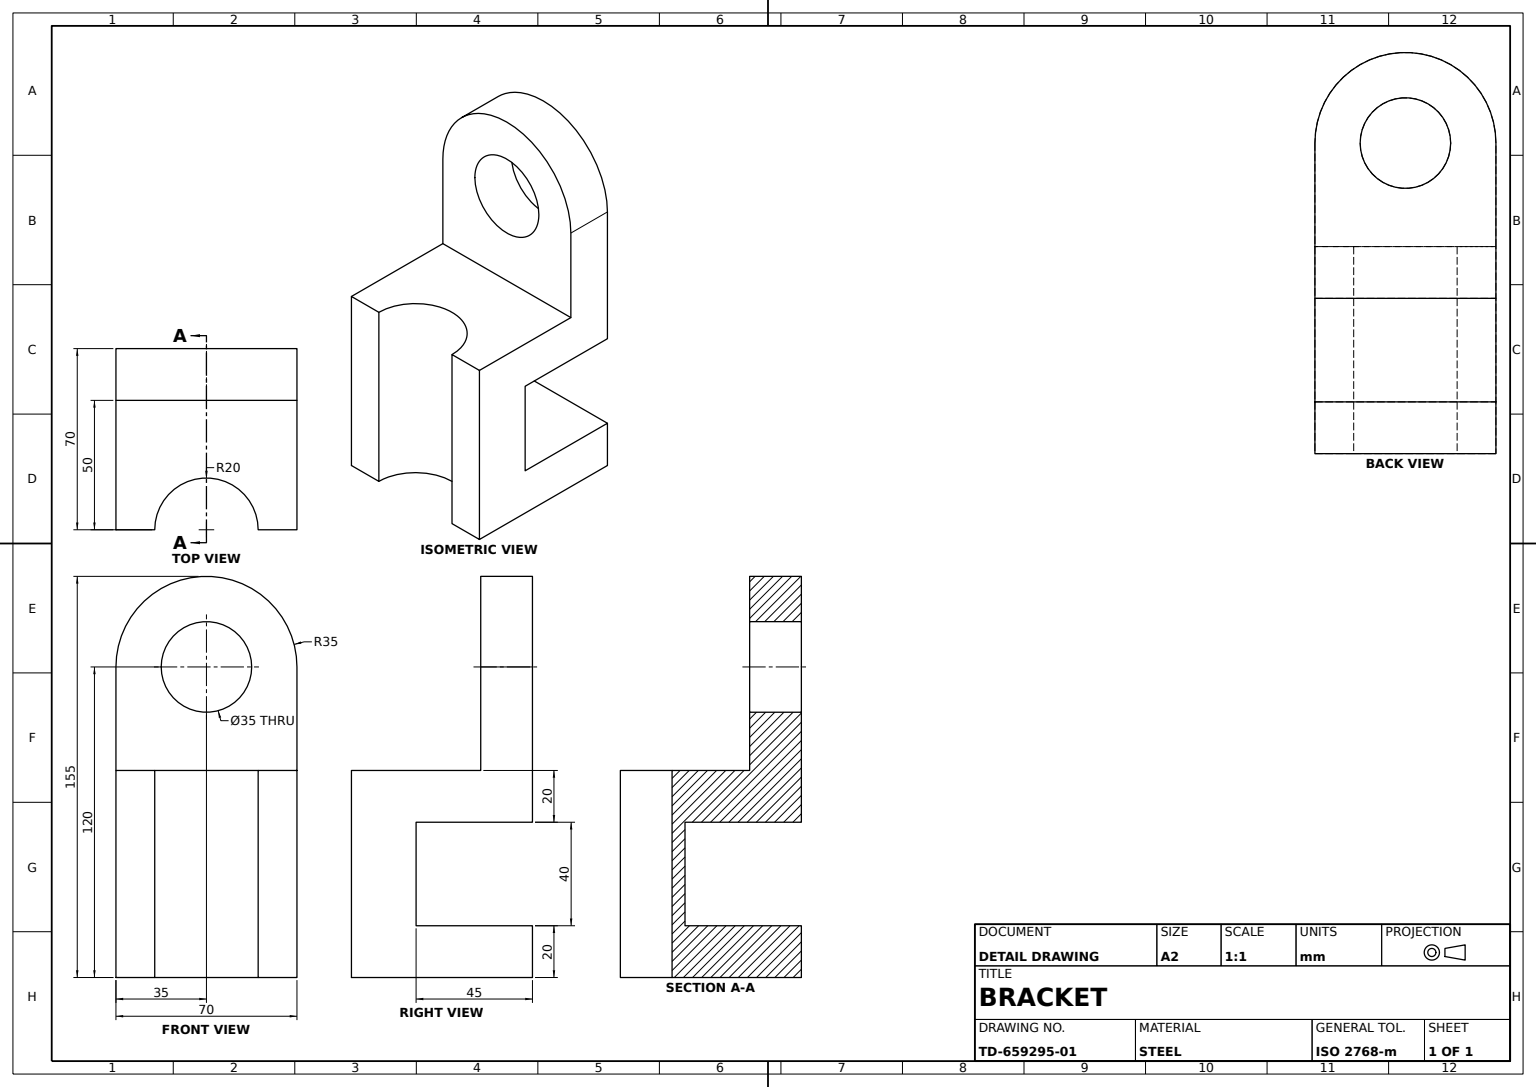
SolidWorks part; units mm, degrees
material "Plain Carbon Steel"
ref_plane "Front Plane" through (0, 0, 0) normal (0, 0, 1) x (1, 0, 0)
ref_plane "Top Plane" through (0, 0, 0) normal (0, 1, 0) x (1, 0, 0)
ref_plane "Right Plane" through (0, 0, 0) normal (1, 0, 0) x (0, 0, -1)
sketch "Base Profile" plane through (0, 0, 0) normal (0, 1, 0) x (1, 0, 0)
  line L6 (35, 0) -> (35, 35)
  line L7 (35, 35) -> (-35, 35)
  line L8 (-35, 35) -> (-35, -35)
  line L9 (-35, -35) -> (35, -35)
  line L10 (35, -35) -> (35, 0)
  dimension "D1" = 70
  dimension "D2" = 70
  dimension "D3" = 35
extrude "Base Block" add sketch "Base Profile" along normal blind 20
sketch "Body Profile" plane through (0, 20, 0) normal (0, 1, 0) x (1, 0, 0)
  line L0 (35, 35) -> (35, -10)
  line L1 (35, -35) -> (35, 35) construction
  line L2 (35, -10) -> (-35, -10)
  line L3 (-35, 35) -> (-35, -35) construction
  line L4 (-35, -10) -> (-35, -35)
  line L5 (-35, -35) -> (35, -35)
  line L6 (35, -35) -> (35, -10)
  line L7 (35, 35) -> (-35, 35) construction
  line M1 (35, -35) -> (35, 35)
  line M3 (-35, 35) -> (-35, -35)
  line M4 (-35, -35) -> (35, -35)
  dimension "D1" = 45
extrude "Body Section" add sketch "Body Profile" along normal blind 40 contours L2 M1 M3 M4
sketch "Shelf Profile" plane through (0, 60, 0) normal (0, 1, 0) x (1, 0, 0)
  line L0 (-35, -35) -> (35, -35)
  line L1 (35, -35) -> (35, 35)
  line L2 (35, 35) -> (-35, 35)
  line L3 (-35, 35) -> (-35, -35)
extrude "Shelf Block" add sketch "Shelf Profile" along normal blind 20
sketch "Upright Profile" plane through (0, 80, 0) normal (0, 1, 0) x (1, 0, 0)
  line L0 (35, 35) -> (35, 15)
  line L1 (35, -35) -> (35, 35) construction
  line L2 (35, 15) -> (-35, 15)
  line L3 (-35, 35) -> (-35, -35) construction
  line L4 (-35, 15) -> (-35, 35)
  line L5 (-35, 35) -> (35, 35)
  dimension "D1" = 50
extrude "Upright Wall" add sketch "Upright Profile" along normal blind 40
sketch "Lug Profile" plane through (0, 0, -15) normal (0, 0, 1) x (1, 0, 0)
  line L0 (-35, 120) -> (35, 120) construction
  line L1 (-35, 120) -> (35, 120)
  arc A0 (35, 120) -> (-35, 120) centre (0, 120) ccw
extrude "Rounded Lug" add sketch "Lug Profile" against normal blind 20
sketch "Lug Hole Profile" plane through (0, 0, -15) normal (0, 0, 1) x (1, 0, 0)
  circle A0 centre (0, 120) radius 17.5
  dimension "D1" = 35
extrude "Lug Through Hole" cut sketch "Lug Hole Profile" against normal blind 208
sketch "Bearing Bore Profile" plane through (0, 80, 0) normal (0, 1, 0) x (1, 0, 0)
  line L0 (-35, -35) -> (35, -35) construction
  line L1 (-20, -35) -> (20, -35)
  arc A0 (20, -35) -> (-20, -35) centre (0, -35) ccw
  dimension "D1" = 20
extrude "Half Bearing Bore" cut sketch "Bearing Bore Profile" against normal blind 208
